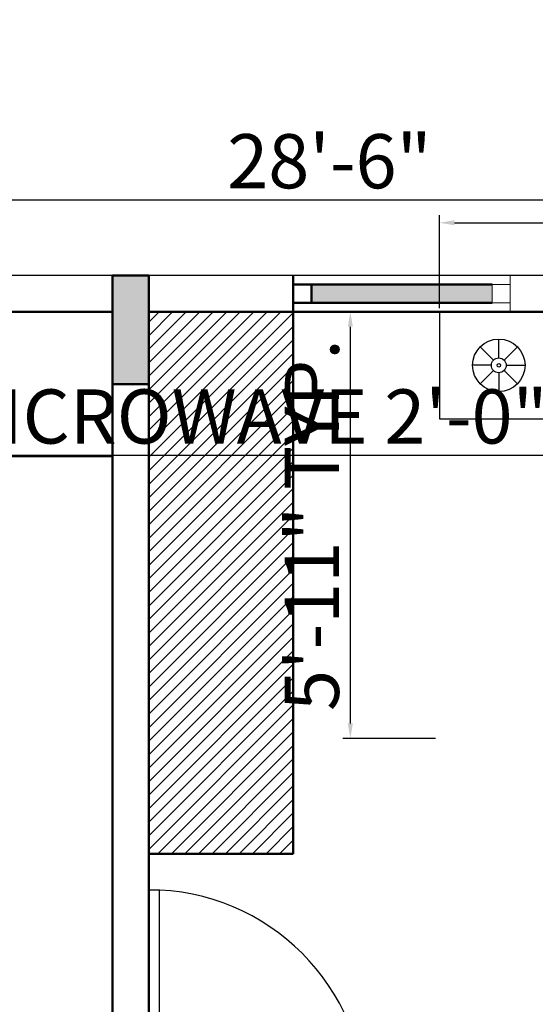
# Model space of a CAD drawing. Units: inches. Extents: x 3064 to 19385, y 846 to 15425.
# Tile 5 of 108: x 3340 to 3426, y 1275 to 1439. Entities that reach past the tile are written whole.
import ezdxf

# ---------------------------------------------------------------- set-up
doc = ezdxf.new("R2010")
doc.units = ezdxf.units.IN
for name, color, linetype, lineweight in [('A-ANNO-DIMS', 2, 'Continuous', 18), ('A-COLS', 1, 'Continuous', 35), ('A-DOOR', 3, 'Continuous', 25), ('A-FLOR-FIXT', 9, 'Continuous', 18), ('A-FURN-PATT', 252, 'Continuous', 13), ('A-GLAZ', 4, 'Continuous', 18), ('A-WALL', 7, 'Continuous', 50), ('C-PROP', 6, 'Continuous', 25)]:
    doc.layers.add(name, color=color, linetype=linetype, lineweight=lineweight)
doc.layers.add('BLOCK', color=6, linetype='Continuous')
doc.styles.get("Standard").update_dxf_attribs({"font": 'arial.ttf'})
doc.dimstyles.new('ISO-25', dxfattribs={"dimtxt": 9, "dimasz": 2.5, "dimexe": 1.25, "dimexo": 0.625, "dimtad": 1, "dimdec": 1, "dimlunit": 3, "dimtxsty": 'Standard', "dimcen": 2.5, "dimadec": 0, "dimazin": 0, "dimtfac": 1, "dimtdec": 1, "dimtmove": 0, "dimatfit": 3, "dimfxl": 1, "dimarcsym": 0})

# ---------------------------------------------------------------- blocks, each defined once
blk = doc.blocks.new('*U3')
for p, q in [((0, 0), (0, -6)), ((36, 0), (36, -6))]:
    blk.add_line(p, q)
blk.add_lwpolyline([(0, 0), (0, 36), (1.75, 36), (1.75, 0)], close=True)
blk.add_arc((0, 0), 36, 0, 90)
blk = doc.blocks.new('A$C52E67D0D')
at = {"layer": 'BLOCK'}
for p, q in [((250.5, 1605.5), (250.5, 1684.7)), ((228.3, 1596.3), (172.3, 1652.3)), ((272.7, 1596.3), (328.7, 1652.3)), ((219.1, 1574.1), (139.9, 1574.1)), ((228.3, 1551.9), (172.3, 1495.9)), ((250.5, 1542.8), (250.5, 1463.5)), ((272.7, 1551.9), (328.7, 1495.9)), ((281.9, 1574.1), (361.1, 1574.1))]:
    blk.add_line(p, q, dxfattribs=at)
blk.add_lwpolyline([(501, 1348.6), (501, 1799.6), (0, 1799.6), (0, 1348.6)], close=True, dxfattribs=at)
for radius in [110.6, 31.4, 7.46]:
    blk.add_circle((250.5, 1574.1), radius, dxfattribs=at)
blk = doc.blocks.new('*D38')
at = {"layer": 'A-ANNO-DIMS', "color": 0, "lineweight": -2, "transparency": 16777216}
for p, q in [((3220.85, 1396.96), (3220.85, 1410.2)), ((3562.85, 1396.96), (3562.85, 1410.2)), ((3223.35, 1408.95), (3560.35, 1408.95))]:
    blk.add_line(p, q, dxfattribs=at)
at = {"layer": 'A-ANNO-DIMS', "color": 0, "transparency": 16777216}
for points in [[(3223.35, 1409.36), (3223.35, 1408.53), (3220.85, 1408.95)], [(3560.35, 1409.36), (3560.35, 1408.53), (3562.85, 1408.95)]]:
    blk.add_solid(points, dxfattribs=at)
at = {"layer": 'Defpoints', "color": 0, "transparency": 16777216}
for p in [(3562.85, 1408.95), (3220.85, 1396.34), (3562.85, 1396.34)]:
    blk.add_point(p, dxfattribs=at)
at = {"layer": 'A-ANNO-DIMS', "color": 0, "transparency": 16777216, "insert": (3391.85, 1414.17), "char_height": 9, "attachment_point": 5}
blk.add_mtext('28\'-6"', dxfattribs=at)
blk = doc.blocks.new('*D401')
at = {"layer": 'A-ANNO-DIMS', "color": 0, "lineweight": -2, "transparency": 16777216}
for p, q in [((3410.1, 1390.96), (3410.1, 1406.37)), ((3508.6, 1390.96), (3508.6, 1406.37)), ((3412.6, 1405.12), (3506.1, 1405.12)), ((3508.6, 1405.12), (3617.13, 1405.12))]:
    blk.add_line(p, q, dxfattribs=at)
at = {"layer": 'A-ANNO-DIMS', "color": 0, "transparency": 16777216}
for points in [[(3412.6, 1405.53), (3412.6, 1404.7), (3410.1, 1405.12)], [(3506.1, 1405.53), (3506.1, 1404.7), (3508.6, 1405.12)]]:
    blk.add_solid(points, dxfattribs=at)
at = {"layer": 'Defpoints', "color": 0, "transparency": 16777216}
for p in [(3508.6, 1405.12), (3410.1, 1390.34), (3508.6, 1390.34)]:
    blk.add_point(p, dxfattribs=at)
at = {"layer": 'A-ANNO-DIMS', "color": 0, "transparency": 16777216, "insert": (3564.11, 1410.39), "char_height": 9, "attachment_point": 5}
blk.add_mtext('BED 8\'-2 1/2" TYP.', dxfattribs=at)
blk = doc.blocks.new('*D402')
at = {"layer": 'A-ANNO-DIMS', "color": 0, "lineweight": -2, "transparency": 16777216}
for p, q in [((3409.47, 1390.34), (3394.07, 1390.34)), ((3395.32, 1321.97), (3395.32, 1387.84)), ((3409.47, 1319.47), (3394.07, 1319.47))]:
    blk.add_line(p, q, dxfattribs=at)
at = {"layer": 'A-ANNO-DIMS', "color": 0, "transparency": 16777216}
for points in [[(3394.9, 1387.84), (3395.74, 1387.84), (3395.32, 1390.34)], [(3394.9, 1321.97), (3395.74, 1321.97), (3395.32, 1319.47)]]:
    blk.add_solid(points, dxfattribs=at)
at = {"layer": 'Defpoints', "color": 0, "transparency": 16777216}
for p in [(3395.32, 1390.34), (3410.1, 1390.34), (3410.1, 1319.47)]:
    blk.add_point(p, dxfattribs=at)
at = {"layer": 'A-ANNO-DIMS', "color": 0, "transparency": 16777216, "insert": (3390.1, 1354.91), "char_height": 9, "attachment_point": 5, "rotation": 90}
blk.add_mtext('5\'-11" TYP.', dxfattribs=at)
blk = doc.blocks.new('*D427')
at = {"layer": 'A-ANNO-DIMS', "color": 0, "lineweight": -2, "transparency": 16777216}
for p, q in [((3296.06, 1369.47), (3296.06, 1365.25)), ((3320.06, 1369.47), (3320.06, 1365.25)), ((3298.56, 1366.5), (3317.56, 1366.5)), ((3320.06, 1366.5), (3460.68, 1366.5))]:
    blk.add_line(p, q, dxfattribs=at)
at = {"layer": 'A-ANNO-DIMS', "color": 0, "transparency": 16777216}
for points in [[(3298.56, 1366.92), (3298.56, 1366.08), (3296.06, 1366.5)], [(3317.56, 1366.92), (3317.56, 1366.08), (3320.06, 1366.5)]]:
    blk.add_solid(points, dxfattribs=at)
at = {"layer": 'Defpoints', "color": 0, "transparency": 16777216}
for p in [(3296.06, 1370.1), (3320.06, 1370.1), (3320.06, 1366.5)]:
    blk.add_point(p, dxfattribs=at)
at = {"layer": 'A-ANNO-DIMS', "color": 0, "transparency": 16777216, "insert": (3391.62, 1371.78), "char_height": 9, "attachment_point": 5}
blk.add_mtext('MICROWAVE 2\'-0" TYP.', dxfattribs=at)

msp = doc.modelspace()

# ---------------------------------------------------------------- hatches: boundary and pattern name
at = {"layer": 'A-COLS'}
h = msp.add_hatch(color=256, dxfattribs=at)
h.dxf.hatch_style = 1
h.paths.add_polyline_path([(3355.85, 1378.34), (3361.85, 1378.34), (3361.85, 1396.34), (3355.85, 1396.34)])
at = {"layer": 'A-FURN-PATT'}
h = msp.add_hatch(dxfattribs=at)
h.set_pattern_fill('ANSI31', color=256, scale=0.5)
h.set_pattern_definition([(45, (-2094.8195, 0), (-1.122532, 1.122532), [])])
h.paths.add_polyline_path([(3385.85, 1390.34), (3361.85, 1390.34), (3361.85, 1378.34), (3361.85, 1300.34), (3385.85, 1300.34)])
at = {"layer": 'A-GLAZ'}
h = msp.add_hatch(color=256, dxfattribs=at)
h.dxf.hatch_style = 1
h.paths.add_polyline_path([(3418.85, 1394.84), (3388.85, 1394.84), (3388.85, 1391.84), (3418.85, 1391.84)])

# ---------------------------------------------------------------- linework, layer by layer
msp.add_line((3421.85, 1396.34), (3421.85, 1390.34), dxfattribs=at)
msp.add_lwpolyline([(3421.85, 1391.84), (3418.85, 1391.84), (3418.85, 1394.84), (3421.85, 1394.84)], close=True, dxfattribs=at)
at = {"layer": 'A-WALL'}
for p, q in [((3385.85, 1396.34), (3385.85, 1390.34)), ((3388.85, 1394.84), (3418.85, 1394.84)), ((3388.85, 1391.84), (3418.85, 1391.84)), ((3355.85, 1390.34), (3226.85, 1390.34)), ((3355.85, 1390.34), (3355.85, 1252.34)), ((3556.85, 1390.34), (3361.85, 1390.34)), ((3361.85, 1390.34), (3361.85, 1252.34)), ((3385.85, 1390.34), (3385.85, 1300.34)), ((3355.85, 1366.34), (3250.85, 1366.34)), ((3385.85, 1300.34), (3361.85, 1300.34))]:
    msp.add_line(p, q, dxfattribs=at)
for points in [[(3361.85, 1378.34), (3361.85, 1396.34), (3355.85, 1396.34), (3355.85, 1378.34)], [(3388.85, 1391.84), (3385.85, 1391.84), (3385.85, 1394.84), (3388.85, 1394.84)]]:
    msp.add_lwpolyline(points, close=True, dxfattribs=at)
at = {"layer": 'C-PROP'}
msp.add_line((3562.85, 1396.34), (3220.85, 1396.34), dxfattribs=at)

# ---------------------------------------------------------------- block references
at = {"layer": 'A-DOOR'}
msp.add_blockref('*U3', (3361.85, 1258.34), dxfattribs=at)
at = {"layer": 'A-FLOR-FIXT', "xscale": 0.039370099999992, "yscale": 0.039370099999992, "zscale": 0.039370099999992}
msp.add_blockref('A$C52E67D0D', (3410.1, 1319.47), dxfattribs=at)

# ---------------------------------------------------------------- dimensions: what is measured, and where the dimension line sits
at = {"layer": 'A-ANNO-DIMS'}
for base, p1, p2, text, picture, middle in [((3508.6, 1405.12), (3410.1, 1390.34), (3508.6, 1390.34), 'BED <> TYP.', '*D401', (3564.11, 1410.39)), ((3320.06, 1366.5), (3296.06, 1370.1), (3320.06, 1370.1), 'MICROWAVE <> TYP.', '*D427', (3391.62, 1371.78))]:
    dim = msp.add_linear_dim(base=base, p1=p1, p2=p2, text=text, dimstyle='ISO-25', override={"dimdec": 1, "dimrnd": 0, "dimzin": 1, "dimlunit": 4, "dimfrac": 2}, dxfattribs=at)
    dim.commit()
    dim.dimension.update_dxf_attribs({"geometry": picture, "text_midpoint": middle})
dim = msp.add_linear_dim(base=(3562.85, 1408.95), p1=(3220.85, 1396.34), p2=(3562.85, 1396.34), dimstyle='ISO-25', override={"dimclrd": 0, "dimclre": 0, "dimclrt": 0}, dxfattribs=at)
dim.commit()
dim.dimension.update_dxf_attribs({"geometry": '*D38', "text_midpoint": (3391.85, 1414.17)})
dim = msp.add_linear_dim(base=(3395.32, 1390.34), p1=(3410.1, 1319.47), p2=(3410.1, 1390.34), angle=90, text='<> TYP.', dimstyle='ISO-25', override={"dimdec": 1, "dimrnd": 0, "dimzin": 1, "dimlunit": 4, "dimfrac": 2}, dxfattribs=at)
dim.commit()
dim.dimension.update_dxf_attribs({"geometry": '*D402', "text_midpoint": (3390.1, 1354.91)})

doc.saveas('drawing.dxf')
